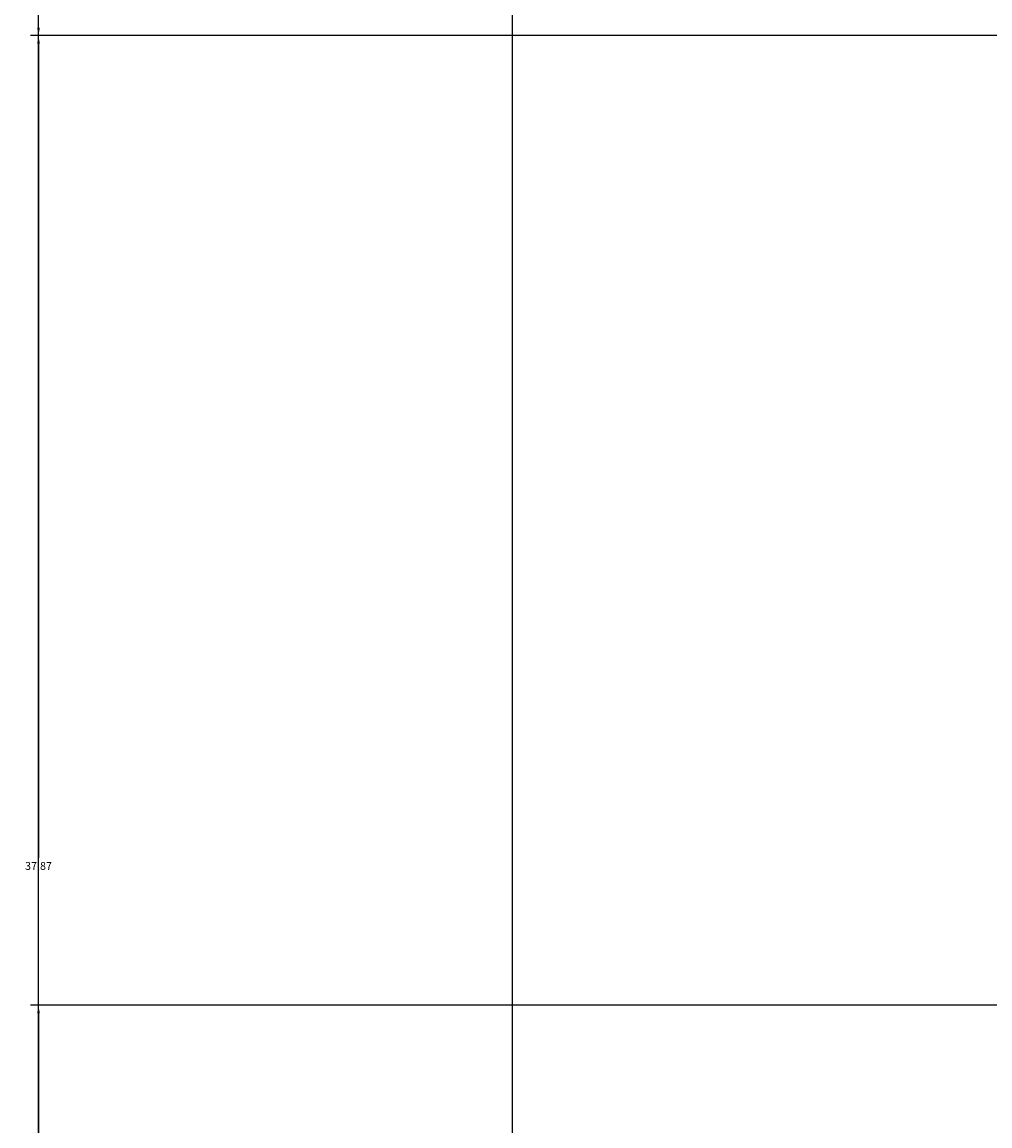
# Model space of a CAD drawing. Units: inches. Extents: x -117 to 121, y -77 to 40.
# Tile 3 of 45: x -117 to -95, y -48 to -23. Entities that reach past the tile are written whole.
import ezdxf

# ---------------------------------------------------------------- set-up
doc = ezdxf.new("R2010")
doc.units = ezdxf.units.IN
doc.header["$MEASUREMENT"] = 0
doc.layers.add('A-ANNO-DIMS', color=2, linetype='Continuous', lineweight=18)
doc.styles.get("Standard").update_dxf_attribs({"font": 'arial.ttf'})
doc.dimstyles.get("Standard").update_dxf_attribs({"dimtxt": 0.18, "dimasz": 0.18, "dimexe": 0.18, "dimexo": 0.0625, "dimgap": 0.09, "dimtad": 0, "dimtih": 1, "dimtoh": 1, "dimdec": 4, "dimzin": 0, "dimdsep": 46, "dimtxsty": 'Standard', "dimcen": 0.09, "dimadec": 0, "dimazin": 0, "dimtfac": 1, "dimtdec": 4, "dimtofl": 0, "dimtmove": 0, "dimatfit": 3, "dimfxl": 1, "dimtolj": 1, "dimtzin": 0, "dimarcsym": 0})

# ---------------------------------------------------------------- blocks, each defined once
blk = doc.blocks.new('*D5')
at = {"layer": 'A-ANNO-DIMS', "color": 0, "lineweight": -2, "transparency": 16777216}
for p, q in [((-94.436, -23.563), (-94.436, -77.193)), ((-106.034, -61.438), (-106.034, -77.193)), ((-105.854, -77.013), (-100.69, -77.013)), ((-94.616, -77.013), (-99.779, -77.013))]:
    blk.add_line(p, q, dxfattribs=at)
at = {"layer": 'A-ANNO-DIMS', "color": 0, "transparency": 16777216}
for points in [[(-105.854, -76.983), (-105.854, -77.043), (-106.034, -77.013)], [(-94.616, -76.983), (-94.616, -77.043), (-94.436, -77.013)]]:
    blk.add_solid(points, dxfattribs=at)
at = {"layer": 'Defpoints', "color": 0, "transparency": 16777216}
for p in [(-94.436, -23.501), (-106.034, -61.376), (-94.436, -77.013)]:
    blk.add_point(p, dxfattribs=at)
at = {"layer": 'A-ANNO-DIMS', "color": 0, "transparency": 16777216, "insert": (-100.235, -77.013), "char_height": 0.18, "attachment_point": 5}
blk.add_mtext('\\A1;11.598', dxfattribs=at)
blk = doc.blocks.new('*D13')
at = {"layer": 'A-ANNO-DIMS', "color": 0, "lineweight": -2, "transparency": 16777216}
for p, q in [((-2.663, 27.063), (-117.024, 27.063)), ((-116.844, 26.883), (-116.844, -16.974)), ((-116.844, -61.196), (-116.844, -17.338)), ((-106.096, -61.376), (-117.024, -61.376))]:
    blk.add_line(p, q, dxfattribs=at)
at = {"layer": 'A-ANNO-DIMS', "color": 0, "transparency": 16777216}
for points in [[(-116.874, 26.883), (-116.814, 26.883), (-116.844, 27.063)], [(-116.874, -61.196), (-116.814, -61.196), (-116.844, -61.376)]]:
    blk.add_solid(points, dxfattribs=at)
at = {"layer": 'Defpoints', "color": 0, "transparency": 16777216}
for p in [(-2.6, 27.063), (-116.844, -61.376), (-106.034, -61.376)]:
    blk.add_point(p, dxfattribs=at)
at = {"layer": 'A-ANNO-DIMS', "color": 0, "transparency": 16777216, "insert": (-116.844, -17.156), "char_height": 0.18, "attachment_point": 5}
blk.add_mtext('\\A1;88.44', dxfattribs=at)
blk = doc.blocks.new('*D18')
at = {"layer": 'A-ANNO-DIMS', "color": 0, "lineweight": -2, "transparency": 16777216}
for p, q in [((-94.498, -23.501), (-117.024, -23.501)), ((-116.844, -23.681), (-116.844, -42.253)), ((-116.844, -61.189), (-116.844, -42.617)), ((-77.826, -61.369), (-117.024, -61.369))]:
    blk.add_line(p, q, dxfattribs=at)
at = {"layer": 'A-ANNO-DIMS', "color": 0, "transparency": 16777216}
for points in [[(-116.874, -23.681), (-116.814, -23.681), (-116.844, -23.501)], [(-116.874, -61.189), (-116.814, -61.189), (-116.844, -61.369)]]:
    blk.add_solid(points, dxfattribs=at)
at = {"layer": 'Defpoints', "color": 0, "transparency": 16777216}
for p in [(-94.436, -23.501), (-116.844, -61.369), (-77.763, -61.369)]:
    blk.add_point(p, dxfattribs=at)
at = {"layer": 'A-ANNO-DIMS', "color": 0, "transparency": 16777216, "insert": (-116.844, -42.435), "char_height": 0.18, "attachment_point": 5}
blk.add_mtext('\\A1;37.87', dxfattribs=at)
blk = doc.blocks.new('*D19')
at = {"layer": 'A-ANNO-DIMS', "color": 0, "lineweight": -2, "transparency": 16777216}
for p, q in [((-94.498, -12.133), (-117.024, -12.133)), ((-116.844, -12.313), (-116.844, -17.635)), ((-116.844, -23.321), (-116.844, -17.999)), ((-94.498, -23.501), (-117.024, -23.501))]:
    blk.add_line(p, q, dxfattribs=at)
at = {"layer": 'A-ANNO-DIMS', "color": 0, "transparency": 16777216}
for points in [[(-116.874, -12.313), (-116.814, -12.313), (-116.844, -12.133)], [(-116.874, -23.321), (-116.814, -23.321), (-116.844, -23.501)]]:
    blk.add_solid(points, dxfattribs=at)
at = {"layer": 'Defpoints', "color": 0, "transparency": 16777216}
for p in [(-94.436, -12.133), (-116.844, -23.501), (-94.436, -23.501)]:
    blk.add_point(p, dxfattribs=at)
at = {"layer": 'A-ANNO-DIMS', "color": 0, "transparency": 16777216, "insert": (-116.844, -17.817), "char_height": 0.18, "attachment_point": 5}
blk.add_mtext('\\A1;11.367', dxfattribs=at)
blk = doc.blocks.new('*D21')
at = {"layer": 'A-ANNO-DIMS', "color": 0, "lineweight": -2, "transparency": 16777216}
for p, q in [((-106.034, -61.313), (-106.034, 38.61)), ((-75.804, 8.087), (-75.804, 38.61)), ((-105.854, 38.43), (-91.382, 38.43)), ((-75.984, 38.43), (-90.455, 38.43))]:
    blk.add_line(p, q, dxfattribs=at)
at = {"layer": 'A-ANNO-DIMS', "color": 0, "transparency": 16777216}
for points in [[(-105.854, 38.46), (-105.854, 38.4), (-106.034, 38.43)], [(-75.984, 38.46), (-75.984, 38.4), (-75.804, 38.43)]]:
    blk.add_solid(points, dxfattribs=at)
at = {"layer": 'Defpoints', "color": 0, "transparency": 16777216}
for p in [(-75.804, 38.43), (-75.804, 8.025), (-106.034, -61.376)]:
    blk.add_point(p, dxfattribs=at)
at = {"layer": 'A-ANNO-DIMS', "color": 0, "transparency": 16777216, "insert": (-90.919, 38.43), "char_height": 0.18, "attachment_point": 5}
blk.add_mtext('\\A1;30.230', dxfattribs=at)
blk = doc.blocks.new('*D37')
at = {"layer": 'A-ANNO-DIMS', "color": 0, "lineweight": -2, "transparency": 16777216}
for p, q in [((-3.912, -45.613), (-117.024, -45.613)), ((-116.844, -45.793), (-116.844, -52.47)), ((-116.844, -59.512), (-116.844, -52.834)), ((-3.912, -59.692), (-117.024, -59.692))]:
    blk.add_line(p, q, dxfattribs=at)
at = {"layer": 'A-ANNO-DIMS', "color": 0, "transparency": 16777216}
for points in [[(-116.874, -45.793), (-116.814, -45.793), (-116.844, -45.613)], [(-116.874, -59.512), (-116.814, -59.512), (-116.844, -59.692)]]:
    blk.add_solid(points, dxfattribs=at)
at = {"layer": 'Defpoints', "color": 0, "transparency": 16777216}
for p in [(-116.844, -45.613), (-3.85, -45.613), (-3.85, -59.692)]:
    blk.add_point(p, dxfattribs=at)
at = {"layer": 'A-ANNO-DIMS', "color": 0, "transparency": 16777216, "insert": (-116.844, -52.652), "char_height": 0.18, "attachment_point": 5}
blk.add_mtext('\\A1;14.079', dxfattribs=at)

msp = doc.modelspace()

# ---------------------------------------------------------------- dimensions: what is measured, and where the dimension line sits
at = {"layer": 'A-ANNO-DIMS'}
for base, p2, picture, middle in [((-75.8037, 38.4297), (-75.8037, 8.0246), '*D21', (-90.9187, 38.4297)), ((-94.4355, -77.0135), (-94.4355, -23.5007), '*D5', (-100.2346, -77.0135))]:
    dim = msp.add_linear_dim(base=base, p1=(-106.0338, -61.3756), p2=p2, dimstyle='Standard', override={"dimdec": 3, "dimlfac": 1, "dimrnd": 0, "dimzin": 0, "dimdsep": 46, "dimlunit": 2}, dxfattribs=at)
    dim.commit()
    dim.dimension.update_dxf_attribs({"geometry": picture, "text_midpoint": middle})
for base, p1, p2, override, picture, middle in [((-116.8438, -61.3756), (-2.6001, 27.0634), (-106.0338, -61.3756), {"dimdec": 2, "dimlfac": 1, "dimrnd": 0, "dimzin": 0, "dimdsep": 46, "dimlunit": 2}, '*D13', (-116.8438, -17.1561)), ((-116.8438, -23.5007), (-94.4355, -12.1334), (-94.4355, -23.5007), {"dimdec": 3, "dimlfac": 1, "dimrnd": 0, "dimzin": 0, "dimdsep": 46, "dimlunit": 2}, '*D19', (-116.8438, -17.817)), ((-116.8438, -61.3689), (-94.4355, -23.5007), (-77.7631, -61.3689), {"dimdec": 2, "dimlfac": 1, "dimrnd": 0, "dimzin": 0, "dimdsep": 46, "dimlunit": 2}, '*D18', (-116.8438, -42.4348)), ((-116.843772, -45.612514), (-3.849514, -59.692012), (-3.849514, -45.612514), {"dimdec": 3, "dimlfac": 1, "dimrnd": 0, "dimzin": 0, "dimdsep": 46, "dimlunit": 2}, '*D37', (-116.843772, -52.652263))]:
    dim = msp.add_linear_dim(base=base, p1=p1, p2=p2, angle=90, dimstyle='Standard', override=override, dxfattribs=at)
    dim.commit()
    dim.dimension.update_dxf_attribs({"geometry": picture, "text_midpoint": middle})

doc.saveas('drawing.dxf')
